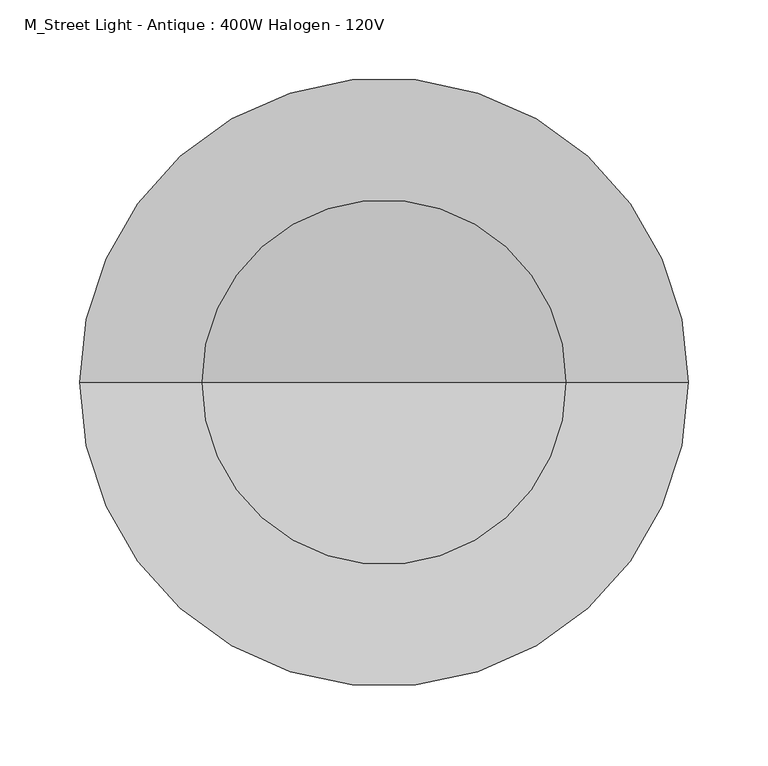
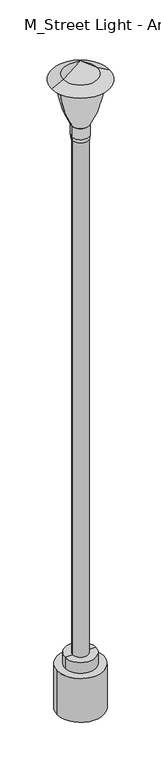
"""IFC4 building model written with IfcOpenShell, lengths in millimetres: light fixture geometry, M_Street Light - Antique : 400W Halogen - 120V."""

from ifc_helpers import new_model, si_unit, point, frame, origin, origin_with_axes, origin_2d, place, context, project, spatial, polyline, circle_curve, ellipse_curve, trimmed, segment, composite_curve, outline, extrude, source, transform, mapped, element, save
from ifc_brep_helpers import plane_surface, cylinder_surface, revolved_surface, advanced_brep


def m_street_light_antique_400w_halogen_120v_ac89fb25(model_context):
    return source(origin(), model_context, "Body", "SolidModel", [
        extrude(outline(composite_curve([segment(trimmed(circle_curve(origin_2d(), 152.4), [point((-152.4, 0.0))], [point((152.4, 0.0))], False, "CARTESIAN"), True, "CONTINUOUS"), segment(trimmed(circle_curve(origin_2d(), 152.4), [point((152.4, 0.0))], [point((-152.4, 0.0))], False, "CARTESIAN"), True, "CONTINUOUS")], self_intersect=False)), origin_with_axes(), (0.0, 0.0, 1.0), 304.8),
        advanced_brep(
        [(190.5, 0.0, 4373.0), (-190.5, 0.0, 4373.0), (-114.3, 0.0, 4411.1), (114.3, 0.0, 4411.1), (114.3, 0.0, 4373.0), (-114.3, 0.0, 4373.0), (114.3, 0.0, 4381.73125), (-114.3, 0.0, 4381.73125), (144.6394367, 0.0, 4381.73125), (-144.6394367, 0.0, 4381.73125), (107.4535144, 0.0, 4400.3242111), (-107.4535144, 0.0, 4400.3242111), (0.0, 0.0, 4485.1715369), (0.0, 0.0, 4500.0)],
        [
            (0, 1, circle_curve(frame((0.0, 0.0, 4373.0), z_axis=(0.0, 0.0, 1.0), x_axis=(-1.0, 0.0, 0.0)), 190.5)),
            (1, 2),
            (2, 3, circle_curve(frame((0.0, 0.0, 4411.1), z_axis=(0.0, 0.0, -1.0), x_axis=(-1.0, 0.0, 0.0)), 114.3)),
            (3, 0),
            (1, 0, circle_curve(frame((0.0, 0.0, 4373.0), z_axis=(0.0, 0.0, 1.0), x_axis=(-1.0, 0.0, 0.0)), 190.5)),
            (3, 2, circle_curve(frame((0.0, 0.0, 4411.1), z_axis=(0.0, 0.0, -1.0), x_axis=(-1.0, 0.0, 0.0)), 114.3)),
            (4, 5, circle_curve(frame((0.0, 0.0, 4373.0), z_axis=(0.0, 0.0, 1.0), x_axis=(-1.0, 0.0, 0.0)), 114.3)),
            (5, 1),
            (0, 4),
            (5, 4, circle_curve(frame((0.0, 0.0, 4373.0), z_axis=(0.0, 0.0, 1.0), x_axis=(-1.0, 0.0, 0.0)), 114.3)),
            (6, 7, circle_curve(frame((0.0, 0.0, 4381.73125), z_axis=(0.0, 0.0, 1.0), x_axis=(-1.0, 0.0, 0.0)), 114.3)),
            (7, 5),
            (4, 6),
            (7, 6, circle_curve(frame((0.0, 0.0, 4381.73125), z_axis=(0.0, 0.0, 1.0), x_axis=(-1.0, 0.0, 0.0)), 114.3)),
            (8, 9, circle_curve(frame((0.0, 0.0, 4381.73125), z_axis=(0.0, 0.0, 1.0), x_axis=(-1.0, 0.0, 0.0)), 144.6394367)),
            (9, 7),
            (6, 8),
            (9, 8, circle_curve(frame((0.0, 0.0, 4381.73125), z_axis=(0.0, 0.0, 1.0), x_axis=(-1.0, 0.0, 0.0)), 144.6394367)),
            (10, 11, circle_curve(frame((0.0, 0.0, 4400.3242111), z_axis=(0.0, 0.0, 1.0), x_axis=(-1.0, 0.0, 0.0)), 107.4535144)),
            (11, 9),
            (8, 10),
            (11, 10, circle_curve(frame((0.0, 0.0, 4400.3242111), z_axis=(0.0, 0.0, 1.0), x_axis=(-1.0, 0.0, 0.0)), 107.4535144)),
            (12, 11),
            (10, 12),
            (2, 13),
            (13, 3),
        ],
        [
            revolved_surface(polyline([(-114.3, 0.0, 4411.1), (-190.5, 0.0, 4373.0)]), (0.0, 0.0, 4754.0), (0.0, 0.0, -1.0)),
            plane_surface(frame((0.0, 0.0, 4373.0), z_axis=(0.0, 0.0, -1.0), x_axis=(-1.0, 0.0, 0.0))),
            revolved_surface(polyline([(-114.3, 0.0, 4373.0), (-114.3, 0.0, 4381.73125)]), (0.0, 0.0, 4754.0), (0.0, 0.0, -1.0)),
            plane_surface(frame((0.0, 0.0, 4381.73125), z_axis=(0.0, 0.0, 1.0), x_axis=(-1.0, 0.0, 0.0))),
            revolved_surface(polyline([(-144.6394367, 0.0, 4381.73125), (-107.4535144, 0.0, 4400.3242111)]), (0.0, 0.0, 4754.0), (0.0, 0.0, -1.0)),
            revolved_surface(polyline([(-107.4535144, 0.0, 4400.3242111), (0.0, 0.0, 4485.1715369)]), (0.0, 0.0, 4754.0), (0.0, 0.0, -1.0)),
            revolved_surface(polyline([(0.0, 0.0, 4500.0), (-114.3, 0.0, 4411.1)]), (0.0, 0.0, 4754.0), (0.0, 0.0, -1.0)),
        ],
        [
            (0, [[1, 2, 3, 4]]),
            (0, [[5, -4, 6, -2]]),
            (1, [[7, 8, -1, 9]]),
            (1, [[10, -9, -5, -8]]),
            (2, [[11, 12, -7, 13]]),
            (2, [[14, -13, -10, -12]]),
            (3, [[15, 16, -11, 17]]),
            (3, [[18, -17, -14, -16]]),
            (4, [[19, 20, -15, 21]]),
            (4, [[22, -21, -18, -20]]),
            (5, [[23, -19, 24]]),
            (5, [[-24, -22, -23]]),
            (6, [[-3, 25, 26]]),
            (6, [[-6, -26, -25]]),
        ],
    ),
        advanced_brep(
        [(53.975, 0.0, 3992.0), (-53.975, 0.0, 3992.0), (-57.3982763, 0.0, 3992.0), (57.3982763, 0.0, 3992.0), (53.975, 0.0, 3966.6), (-53.975, 0.0, 3966.6), (12.7, 0.0, 3966.6), (-12.7, 0.0, 3966.6), (12.7, 0.0, 3992.0), (-12.7, 0.0, 3992.0), (31.9982763, 0.0, 3992.0), (-31.9982763, 0.0, 3992.0), (31.9982763, 0.0, 4068.2), (-31.9982763, 0.0, 4068.2), (57.3982763, 0.0, 4068.2), (-57.3982763, 0.0, 4068.2)],
        [
            (0, 1, circle_curve(frame((0.0, 0.0, 3992.0), z_axis=(0.0, 0.0, 1.0), x_axis=(-1.0, 0.0, 0.0)), 53.975)),
            (1, 2),
            (2, 3, circle_curve(frame((0.0, 0.0, 3992.0), z_axis=(0.0, 0.0, -1.0), x_axis=(-1.0, 0.0, 0.0)), 57.3982763)),
            (3, 0),
            (1, 0, circle_curve(frame((0.0, 0.0, 3992.0), z_axis=(0.0, 0.0, 1.0), x_axis=(-1.0, 0.0, 0.0)), 53.975)),
            (3, 2, circle_curve(frame((0.0, 0.0, 3992.0), z_axis=(0.0, 0.0, -1.0), x_axis=(-1.0, 0.0, 0.0)), 57.3982763)),
            (4, 5, circle_curve(frame((0.0, 0.0, 3966.6), z_axis=(0.0, 0.0, 1.0), x_axis=(-1.0, 0.0, 0.0)), 53.975)),
            (5, 1),
            (0, 4),
            (5, 4, circle_curve(frame((0.0, 0.0, 3966.6), z_axis=(0.0, 0.0, 1.0), x_axis=(-1.0, 0.0, 0.0)), 53.975)),
            (6, 7, circle_curve(frame((0.0, 0.0, 3966.6), z_axis=(0.0, 0.0, 1.0), x_axis=(-1.0, 0.0, 0.0)), 12.7)),
            (7, 5),
            (4, 6),
            (7, 6, circle_curve(frame((0.0, 0.0, 3966.6), z_axis=(0.0, 0.0, 1.0), x_axis=(-1.0, 0.0, 0.0)), 12.7)),
            (8, 9, circle_curve(frame((0.0, 0.0, 3992.0), z_axis=(0.0, 0.0, 1.0), x_axis=(-1.0, 0.0, 0.0)), 12.7)),
            (9, 7),
            (6, 8),
            (9, 8, circle_curve(frame((0.0, 0.0, 3992.0), z_axis=(0.0, 0.0, 1.0), x_axis=(-1.0, 0.0, 0.0)), 12.7)),
            (10, 11, circle_curve(frame((0.0, 0.0, 3992.0), z_axis=(0.0, 0.0, 1.0), x_axis=(-1.0, 0.0, 0.0)), 31.9982763)),
            (11, 9),
            (8, 10),
            (11, 10, circle_curve(frame((0.0, 0.0, 3992.0), z_axis=(0.0, 0.0, 1.0), x_axis=(-1.0, 0.0, 0.0)), 31.9982763)),
            (12, 13, circle_curve(frame((0.0, 0.0, 4068.2), z_axis=(0.0, 0.0, 1.0), x_axis=(-1.0, 0.0, 0.0)), 31.9982763)),
            (13, 11),
            (10, 12),
            (13, 12, circle_curve(frame((0.0, 0.0, 4068.2), z_axis=(0.0, 0.0, 1.0), x_axis=(-1.0, 0.0, 0.0)), 31.9982763)),
            (14, 15, circle_curve(frame((0.0, 0.0, 4068.2), z_axis=(0.0, 0.0, 1.0), x_axis=(-1.0, 0.0, 0.0)), 57.3982763)),
            (15, 13),
            (12, 14),
            (15, 14, circle_curve(frame((0.0, 0.0, 4068.2), z_axis=(0.0, 0.0, 1.0), x_axis=(-1.0, 0.0, 0.0)), 57.3982763)),
            (2, 15),
            (14, 3),
        ],
        [
            plane_surface(frame((0.0, 0.0, 3992.0), z_axis=(0.0, 0.0, -1.0), x_axis=(-1.0, 0.0, 0.0))),
            cylinder_surface(frame((0.0, 0.0, 4754.0), z_axis=(0.0, 0.0, -1.0), x_axis=(-1.0, 0.0, 0.0)), 53.975),
            plane_surface(frame((0.0, 0.0, 3966.6), z_axis=(0.0, 0.0, -1.0), x_axis=(-1.0, 0.0, 0.0))),
            revolved_surface(polyline([(-12.7, 0.0, 3966.6), (-12.7, 0.0, 3992.0)]), (0.0, 0.0, 4754.0), (0.0, 0.0, -1.0)),
            plane_surface(frame((0.0, 0.0, 3992.0), z_axis=(0.0, 0.0, 1.0), x_axis=(-1.0, 0.0, 0.0))),
            revolved_surface(polyline([(-31.9982763, 0.0, 3992.0), (-31.9982763, 0.0, 4068.2)]), (0.0, 0.0, 4754.0), (0.0, 0.0, -1.0)),
            plane_surface(frame((0.0, 0.0, 4068.2), z_axis=(0.0, 0.0, 1.0), x_axis=(-1.0, 0.0, 0.0))),
            cylinder_surface(frame((0.0, 0.0, 4754.0), z_axis=(0.0, 0.0, -1.0), x_axis=(-1.0, 0.0, 0.0)), 57.3982763),
        ],
        [
            (0, [[1, 2, 3, 4]]),
            (0, [[5, -4, 6, -2]]),
            (1, [[7, 8, -1, 9]]),
            (1, [[10, -9, -5, -8]]),
            (2, [[11, 12, -7, 13]]),
            (2, [[14, -13, -10, -12]]),
            (3, [[15, 16, -11, 17]]),
            (3, [[18, -17, -14, -16]]),
            (4, [[19, 20, -15, 21]]),
            (4, [[22, -21, -18, -20]]),
            (5, [[23, 24, -19, 25]]),
            (5, [[26, -25, -22, -24]]),
            (6, [[27, 28, -23, 29]]),
            (6, [[30, -29, -26, -28]]),
            (7, [[-3, 31, -27, 32]]),
            (7, [[-6, -32, -30, -31]]),
        ],
    ),
        advanced_brep(
        [(101.6, 0.0, 381.0), (-101.6, 0.0, 381.0), (-101.6, 0.0, 304.8), (101.6, 0.0, 304.8), (50.8, 0.0, 381.0), (-50.8, 0.0, 381.0), (50.8, 0.0, 3966.6), (-50.8, 0.0, 3966.6), (25.4, 0.0, 3966.6), (-25.4, 0.0, 3966.6), (25.4, 0.0, 304.8), (-25.4, 0.0, 304.8)],
        [
            (0, 1, circle_curve(frame((0.0, 0.0, 381.0), z_axis=(0.0, 0.0, -1.0), x_axis=(-1.0, 0.0, 0.0)), 101.6)),
            (1, 2),
            (2, 3, circle_curve(frame((0.0, 0.0, 304.8), z_axis=(0.0, 0.0, 1.0), x_axis=(-1.0, 0.0, 0.0)), 101.6)),
            (3, 0),
            (4, 5, circle_curve(frame((0.0, 0.0, 381.0), z_axis=(0.0, 0.0, -1.0), x_axis=(-1.0, 0.0, 0.0)), 50.8)),
            (5, 1),
            (0, 4),
            (6, 7, circle_curve(frame((0.0, 0.0, 3966.6), z_axis=(0.0, 0.0, -1.0), x_axis=(-1.0, 0.0, 0.0)), 50.8)),
            (7, 5),
            (4, 6),
            (8, 9, circle_curve(frame((0.0, 0.0, 3966.6), z_axis=(0.0, 0.0, -1.0), x_axis=(-1.0, 0.0, 0.0)), 25.4)),
            (9, 7),
            (6, 8),
            (10, 11, circle_curve(frame((0.0, 0.0, 304.8), z_axis=(0.0, 0.0, -1.0), x_axis=(-1.0, 0.0, 0.0)), 25.4)),
            (11, 9),
            (8, 10),
            (2, 11),
            (10, 3),
            (1, 0, circle_curve(frame((0.0, 0.0, 381.0), z_axis=(0.0, 0.0, -1.0), x_axis=(1.0, 0.0, 0.0)), 101.6)),
            (3, 2, circle_curve(frame((0.0, 0.0, 304.8), z_axis=(0.0, 0.0, 1.0), x_axis=(1.0, 0.0, 0.0)), 101.6)),
            (5, 4, circle_curve(frame((0.0, 0.0, 381.0), z_axis=(0.0, 0.0, -1.0), x_axis=(1.0, 0.0, 0.0)), 50.8)),
            (7, 6, circle_curve(frame((0.0, 0.0, 3966.6), z_axis=(0.0, 0.0, -1.0), x_axis=(1.0, 0.0, 0.0)), 50.8)),
            (9, 8, circle_curve(frame((0.0, 0.0, 3966.6), z_axis=(0.0, 0.0, -1.0), x_axis=(1.0, 0.0, 0.0)), 25.4)),
            (11, 10, circle_curve(frame((0.0, 0.0, 304.8), z_axis=(0.0, 0.0, -1.0), x_axis=(1.0, 0.0, 0.0)), 25.4)),
        ],
        [
            cylinder_surface(frame((0.0, 0.0, 304.8), z_axis=(0.0, 0.0, 1.0), x_axis=(-1.0, 0.0, 0.0)), 101.6),
            plane_surface(frame((0.0, 0.0, 381.0), z_axis=(0.0, 0.0, 1.0), x_axis=(-1.0, 0.0, 0.0))),
            cylinder_surface(frame((0.0, 0.0, 304.8), z_axis=(0.0, 0.0, 1.0), x_axis=(-1.0, 0.0, 0.0)), 50.8),
            plane_surface(frame((0.0, 0.0, 3966.6), z_axis=(0.0, 0.0, 1.0), x_axis=(-1.0, 0.0, 0.0))),
            revolved_surface(polyline([(-25.4, 0.0, 3966.6), (-25.4, 0.0, 304.8)]), (0.0, 0.0, 304.8), (0.0, 0.0, 1.0)),
            plane_surface(frame((0.0, 0.0, 304.8), z_axis=(0.0, 0.0, -1.0), x_axis=(-1.0, 0.0, 0.0))),
            cylinder_surface(frame((0.0, 0.0, 304.8), z_axis=(0.0, 0.0, 1.0), x_axis=(1.0, 0.0, 0.0)), 101.6),
            plane_surface(frame((0.0, 0.0, 381.0), z_axis=(0.0, 0.0, 1.0), x_axis=(1.0, 0.0, 0.0))),
            cylinder_surface(frame((0.0, 0.0, 304.8), z_axis=(0.0, 0.0, 1.0), x_axis=(1.0, 0.0, 0.0)), 50.8),
            plane_surface(frame((0.0, 0.0, 3966.6), z_axis=(0.0, 0.0, 1.0), x_axis=(1.0, 0.0, 0.0))),
            revolved_surface(polyline([(25.4, 0.0, 3966.6), (25.4, 0.0, 304.8)]), (0.0, 0.0, 304.8), (0.0, 0.0, 1.0)),
            plane_surface(frame((0.0, 0.0, 304.8), z_axis=(0.0, 0.0, -1.0), x_axis=(1.0, 0.0, 0.0))),
        ],
        [
            (0, [[1, 2, 3, 4]]),
            (1, [[5, 6, -1, 7]]),
            (2, [[8, 9, -5, 10]]),
            (3, [[11, 12, -8, 13]]),
            (4, [[14, 15, -11, 16]]),
            (5, [[-3, 17, -14, 18]]),
            (6, [[19, -4, 20, -2]]),
            (7, [[21, -7, -19, -6]]),
            (8, [[22, -10, -21, -9]]),
            (9, [[23, -13, -22, -12]]),
            (10, [[24, -16, -23, -15]]),
            (11, [[-20, -18, -24, -17]]),
        ],
    ),
        advanced_brep(
        [(57.3982763, 0.0, 4068.2), (-57.3982763, 0.0, 4068.2), (-139.0691901, 0.0, 4373.0), (139.0691901, 0.0, 4373.0), (51.0432576, 0.0, 4068.2), (-51.0432576, 0.0, 4068.2), (131.8784122, 0.0, 4373.0), (-131.8784122, 0.0, 4373.0)],
        [
            (0, 1, circle_curve(frame((0.0, 0.0, 4068.2), z_axis=(0.0, 0.0, 1.0), x_axis=(-1.0, 0.0, 0.0)), 57.3982763)),
            (1, 2, circle_curve(frame((555.9362168, 0.0, 4395.8843098), z_axis=(0.0, 1.0, 0.0), x_axis=(1.0, 0.0, 0.0)), 695.3820586)),
            (2, 3, circle_curve(frame((0.0, 0.0, 4373.0), z_axis=(0.0, 0.0, -1.0), x_axis=(-1.0, 0.0, 0.0)), 139.0691901)),
            (3, 0, circle_curve(frame((-555.9362168, 0.0, 4395.8843098), z_axis=(0.0, 1.0, 0.0), x_axis=(-1.0, 0.0, 0.0)), 695.3820586)),
            (1, 0, circle_curve(frame((0.0, 0.0, 4068.2), z_axis=(0.0, 0.0, 1.0), x_axis=(-1.0, 0.0, 0.0)), 57.3982763)),
            (3, 2, circle_curve(frame((0.0, 0.0, 4373.0), z_axis=(0.0, 0.0, -1.0), x_axis=(-1.0, 0.0, 0.0)), 139.0691901)),
            (4, 5, circle_curve(frame((0.0, 0.0, 4068.2), z_axis=(0.0, 0.0, 1.0), x_axis=(-1.0, 0.0, 0.0)), 51.0432576)),
            (5, 1),
            (0, 4),
            (5, 4, circle_curve(frame((0.0, 0.0, 4068.2), z_axis=(0.0, 0.0, 1.0), x_axis=(-1.0, 0.0, 0.0)), 51.0432576)),
            (6, 7, circle_curve(frame((0.0, 0.0, 4373.0), z_axis=(0.0, 0.0, 1.0), x_axis=(-1.0, 0.0, 0.0)), 131.8784122)),
            (7, 5, circle_curve(frame((563.1799394, 0.0, 4394.2154469), z_axis=(0.0, -1.0, 0.0), x_axis=(1.0, 0.0, 0.0)), 695.3820586)),
            (4, 6, circle_curve(frame((-563.1799394, 0.0, 4394.2154469), z_axis=(0.0, -1.0, 0.0), x_axis=(-1.0, 0.0, 0.0)), 695.3820586)),
            (7, 6, circle_curve(frame((0.0, 0.0, 4373.0), z_axis=(0.0, 0.0, 1.0), x_axis=(-1.0, 0.0, 0.0)), 131.8784122)),
            (2, 7),
            (6, 3),
        ],
        [
            revolved_surface(trimmed(ellipse_curve(frame((555.9362168, 0.0, 4395.8843098), z_axis=(0.0, -1.0, 0.0), x_axis=(1.0, 0.0, 0.0)), 695.3820586, 695.3820586), [point((-139.0691901, 0.0, 4373.0))], [point((-57.3982763, 0.0, 4068.2))], True, "CARTESIAN"), (0.0, 0.0, 4677.8), (0.0, 0.0, -1.0)),
            plane_surface(frame((0.0, 0.0, 4068.2), z_axis=(0.0, 0.0, -1.0), x_axis=(-1.0, 0.0, 0.0))),
            revolved_surface(trimmed(ellipse_curve(frame((563.1799394, 0.0, 4394.2154469), z_axis=(0.0, 1.0, 0.0), x_axis=(1.0, 0.0, 0.0)), 695.3820586, 695.3820586), [point((-51.0432576, 0.0, 4068.2))], [point((-131.8784122, 0.0, 4373.0))], True, "CARTESIAN"), (0.0, 0.0, 4677.8), (0.0, 0.0, -1.0)),
            plane_surface(frame((0.0, 0.0, 4373.0), z_axis=(0.0, 0.0, 1.0), x_axis=(-1.0, 0.0, 0.0))),
        ],
        [
            (0, [[1, 2, 3, 4]]),
            (0, [[5, -4, 6, -2]]),
            (1, [[7, 8, -1, 9]]),
            (1, [[10, -9, -5, -8]]),
            (2, [[11, 12, -7, 13]]),
            (2, [[14, -13, -10, -12]]),
            (3, [[-3, 15, -11, 16]]),
            (3, [[-6, -16, -14, -15]]),
        ],
    ),
    ])


if __name__ == "__main__":
    model = new_model("IFC4")
    model_context = context("Model", 3, world=origin())
    ifc_project = project(units=[si_unit("LENGTHUNIT", "METRE", prefix="MILLI")], contexts=[model_context])
    site = spatial("IfcSite", under=ifc_project)
    building = spatial("IfcBuilding", under=site)
    placement = place(None, origin())
    m_street_light_antique_400w_halogen_120v_shape = m_street_light_antique_400w_halogen_120v_ac89fb25(model_context)
    element("IfcLightFixture", 1, ObjectType="M_Street Light - Antique : 400W Halogen - 120V", at=placement, inside=building, context=model_context, shape_type="MappedRepresentation", body=[
        mapped(m_street_light_antique_400w_halogen_120v_shape, transform((0.0, 0.0, 0.0), x_axis=(1.0, 0.0, 0.0), y_axis=(0.0, 1.0, 0.0), z_axis=(0.0, 0.0, 1.0))),
    ])
    save(model, "model.ifc")

# Revit data of these elements
# Type "M_Street Light - Antique : 400W Halogen - 120V"
#   Photometric Web File = "SLS1T3.ies"
#   Assembly Code = "D5020280"
#   Lamp = "T-3"
#   Wattage Comments = "400"
#   Wattage = 400 W
#   built-in parameter 1150110 = 1 (stored number, unit not read)
#   built-in parameter 1114217 = 1 (stored number, unit not read)
#   built-in parameter 1150109 = 1 (stored number, unit not read)
#   built-in parameter 1150113 = 1 (stored number, unit not read)
#   Tilt Angle = -90.00°
#   built-in parameter 1150115 = 1 (stored number, unit not read)
#   built-in parameter 1150105 = 795.775 (stored number, unit not read)
#   built-in parameter 1150112 = 1 (stored number, unit not read)
#   built-in parameter 1150114 = 1 (stored number, unit not read)
#   built-in parameter 1150107 = 6500 (stored number, unit not read)
#   built-in parameter 1150106 = 7.95775 (stored number, unit not read)
#   built-in parameter 1150104 = 2.32258 (stored number, unit not read)
#   Ballast Voltage = 120 V
#   built-in parameter 1114218 = 1 (stored number, unit not read)
#   built-in parameter 1150133 = 10 (stored number, unit not read)
#   Height = 14' - 9.16535"
#   Lumens = 10000 lm
#   Apparent Load = 400 VA
#   built-in parameter 1150134 = 1
#   built-in parameter 1150137 = 1
#   Color Filter = 16777215
#   Ballast Number of Poles = 1
#   Load Classification = Lighting - Exterior
#   Shade Material = Glass, Frosted
#   Stand Material = Steel, Paint Finish, Dark Gray, Matte
#   Dimming Lamp Color Temperature Shift = (empty or 0)
#   Default Elevation = 0
# Element 1 (IfcLightFixture, "M_Street Light - Antique : 400W Halogen - 120V")
#   Materials on its faces: "Steel, Paint Finish, Dark Gray, Matte", "Glass, Frosted"
# Materials
#   "Glass, Frosted": class "Glass", colour RGB 250 244 225, transparency 0.55, Description = "physical material", Cost = 0
#   "Steel, Paint Finish, Dark Gray, Matte": class "Metal", colour RGB 98 98 98, transparency 0, Description = "Steel, paint finish, dark gray, matte", Cost = 0
